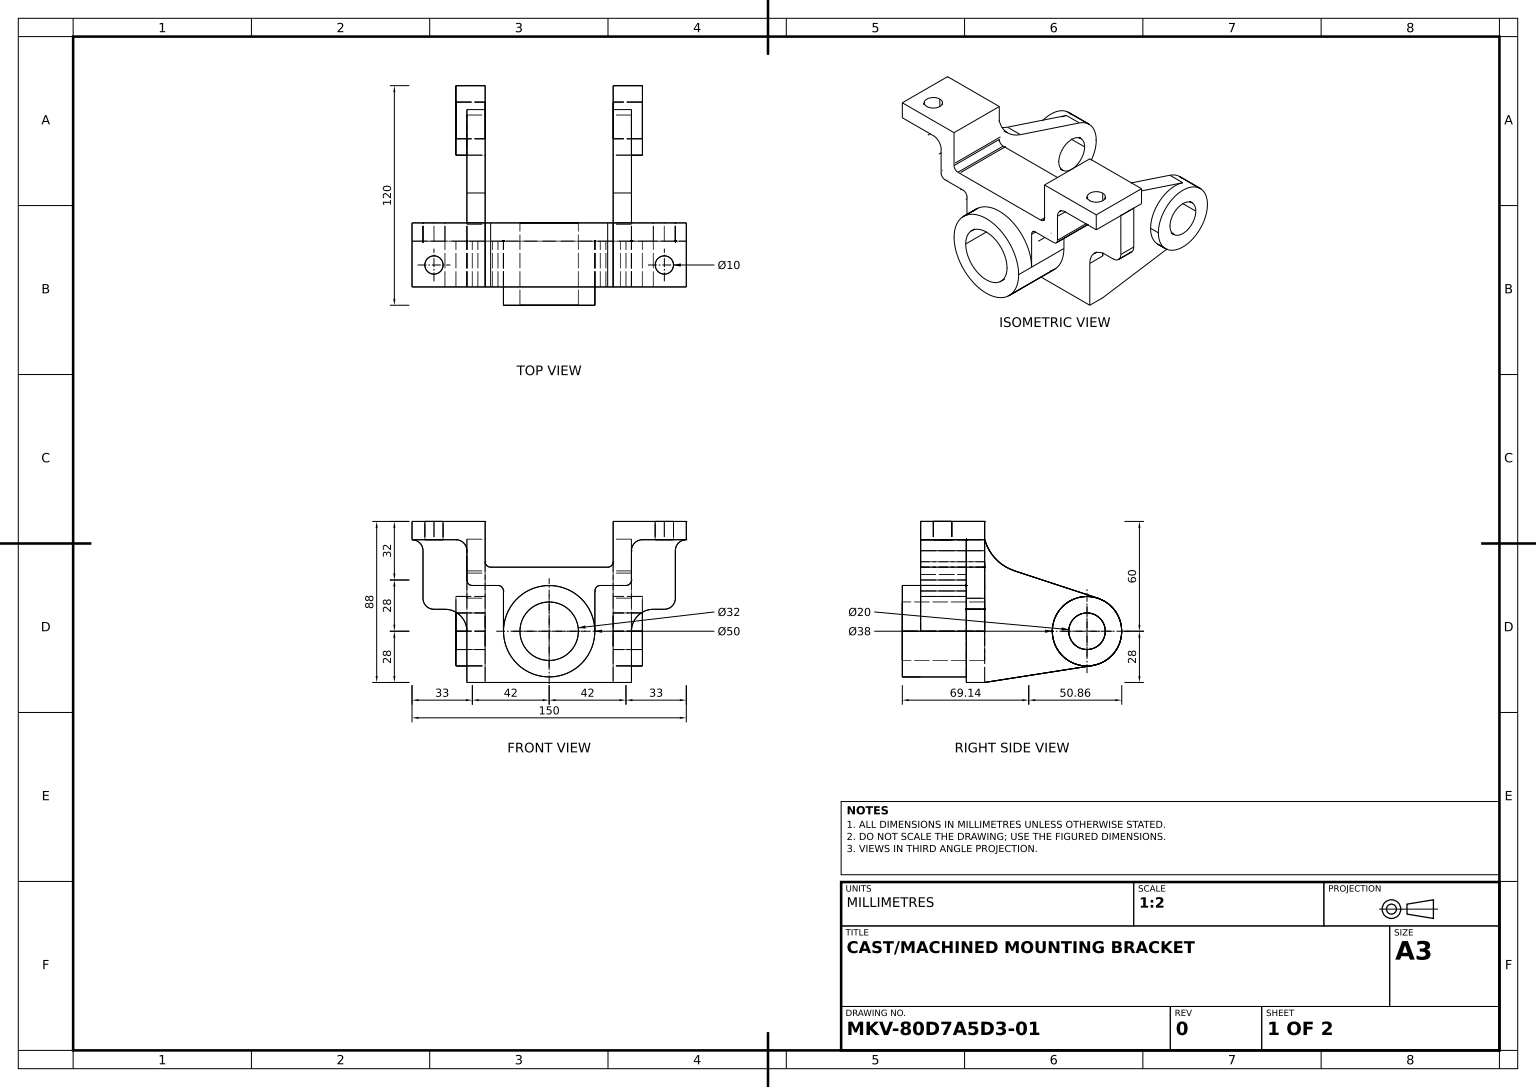
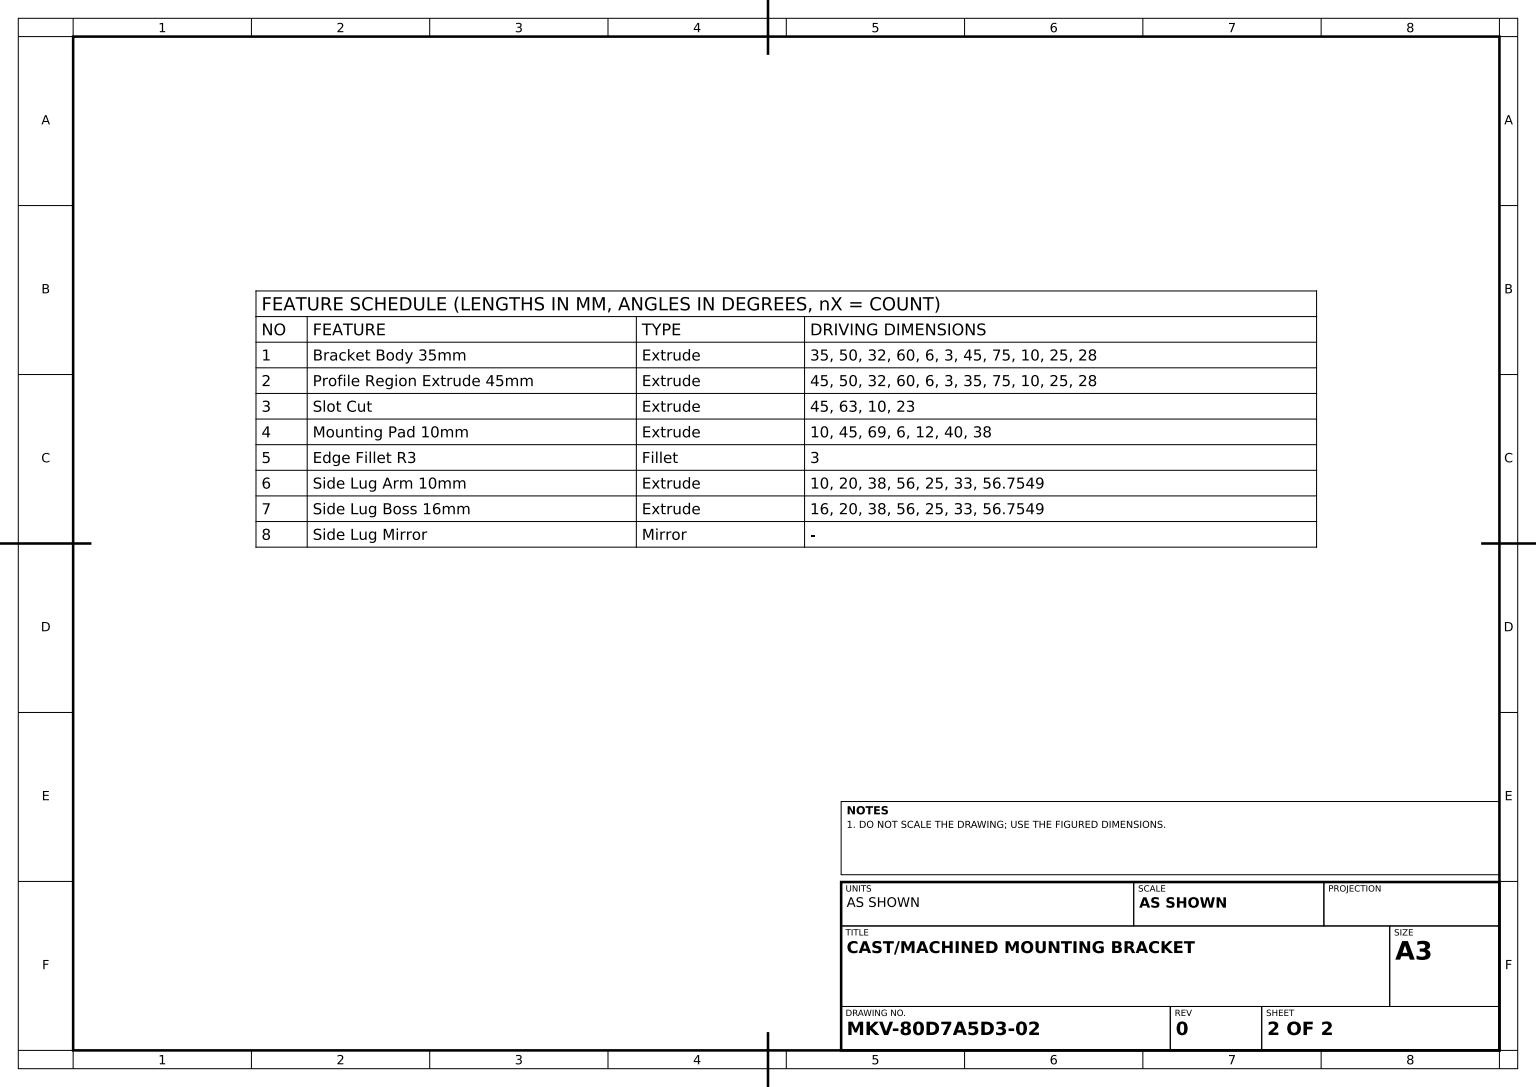
from build123d import *

# Parameters (mm, degrees)
BRACKET_BODY_35MM_DEPTH           = 35
PROFILE_REGION_EXTRUDE_45MM_DEPTH = 45
SLOT_CUT_SKETCH_R                 = 5
SLOT_CUT_DEPTH                    = 45
MOUNTING_PAD_10MM_DEPTH           = 10
EDGE_FILLET_R3_R                  = 3
SIDE_LUG_ARM_10MM_DEPTH           = 10
SKETCH6_3_R                       = 19
SKETCH6_3_R_2                     = 10
SIDE_LUG_BOSS_16MM_DEPTH          = 16


with BuildPart() as part:
    # Bracket Profile Sketch → Bracket Body 35mm (new body)
    with BuildSketch(Plane.XY):
        with BuildLine():
            Line((0, 35), (0, 25))
            ThreePointArc((0, 25), (17.67766953, 17.67766953), (25, 0))
            Line((25, 0), (25, 22))
            ThreePointArc((25, 22), (25.878679656, 24.121320344), (28, 25))
            Line((28, 25), (42, 25))
            ThreePointArc((42, 25), (44.121320344, 25.878679656), (45, 28))
            Line((45, 28), (45, 44))
            ThreePointArc((45, 44), (46.757359313, 48.242640687), (51, 50))
            Line((51, 50), (75, 50))
            Line((75, 50), (75, 60))
            Line((75, 60), (35, 60))
            Line((35, 60), (35, 35))
            Line((35, 35), (0, 35))
        make_face()
        with BuildLine():
            Line((-25, 22), (-25, 0))
            ThreePointArc((-25, 0), (-17.67766953, 17.67766953), (0, 25))
            Line((0, 25), (0, 35))
            Line((0, 35), (-35, 35))
            Line((-35, 35), (-35, 60))
            Line((-35, 60), (-75, 60))
            Line((-75, 60), (-75, 50))
            Line((-75, 50), (-51, 50))
            ThreePointArc((-51, 50), (-46.757359313, 48.242640687), (-45, 44))
            Line((-45, 44), (-45, 28))
            ThreePointArc((-45, 28), (-44.121320344, 25.878679656), (-42, 25))
            Line((-42, 25), (-28, 25))
            ThreePointArc((-28, 25), (-25.878679656, 24.121320344), (-25, 22))
        make_face()
    extrude(amount=BRACKET_BODY_35MM_DEPTH)

    # Sketch1_3 → Profile Region Extrude 45mm (add)
    with BuildSketch(Plane.XY):
        with BuildLine():
            ThreePointArc((0, 25), (-17.67766953, 17.67766953), (-25, 0))
            ThreePointArc((-25, 0), (-17.67766953, -17.67766953), (0, -25))
            Line((0, -25), (0, -16))
            ThreePointArc((0, -16), (-16, 0), (0, 16))
            Line((0, 16), (0, 25))
        make_face()
        with BuildLine():
            ThreePointArc((25, 0), (17.67766953, 17.67766953), (0, 25))
            Line((0, 25), (0, 16))
            ThreePointArc((0, 16), (11.313708499, 11.313708499), (16, 0))
            ThreePointArc((16, 0), (11.313708499, -11.313708499), (0, -16))
            Line((0, -16), (0, -25))
            ThreePointArc((0, -25), (17.67766953, -17.67766953), (25, 0))
        make_face()
        with BuildLine():
            ThreePointArc((0, 25), (-17.67766953, 17.67766953), (-25, 0))
            ThreePointArc((-25, 0), (-17.67766953, -17.67766953), (0, -25))
            Line((0, -25), (0, -16))
            ThreePointArc((0, -16), (-16, 0), (0, 16))
            Line((0, 16), (0, 25))
        make_face()
        with BuildLine():
            ThreePointArc((25, 0), (17.67766953, 17.67766953), (0, 25))
            Line((0, 25), (0, 16))
            ThreePointArc((0, 16), (11.313708499, 11.313708499), (16, 0))
            ThreePointArc((16, 0), (11.313708499, -11.313708499), (0, -16))
            Line((0, -16), (0, -25))
            ThreePointArc((0, -25), (17.67766953, -17.67766953), (25, 0))
        make_face()
    extrude(amount=PROFILE_REGION_EXTRUDE_45MM_DEPTH)

    # Slot Cut Sketch → Slot Cut (cut)
    with BuildSketch(Plane.XZ.offset(-50)):
        with Locations(Location((63, 23, 0), (0, 0, 270))):
            Circle(SLOT_CUT_SKETCH_R)
        with Locations(Location((-63, 23, 0), (0, 0, 270))):
            Circle(SLOT_CUT_SKETCH_R)
    extrude(amount=-SLOT_CUT_DEPTH, mode=Mode.SUBTRACT)

    # Mounting Pad Sketch → Mounting Pad 10mm (add)
    with BuildSketch(Plane(origin=(0, 0, 0), x_dir=(-1, 0, 0), z_dir=(0, 0, -1))):
        with BuildLine():
            Line((51, 50), (75, 50))
            ThreePointArc((75, 50), (70.757359313, 48.242640687), (69, 44))
            Line((69, 44), (69, 18))
            ThreePointArc((69, 18), (67.242640687, 13.757359313), (63, 12))
            Line((63, 12), (57, 12))
            ThreePointArc((57, 12), (48.514718626, 8.485281374), (45, 0))
            Line((45, 0), (45, -28))
            Line((45, -28), (-45, -28))
            Line((-45, -28), (-45, 0))
            ThreePointArc((-45, 0), (-48.514718626, 8.485281374), (-57, 12))
            Line((-57, 12), (-63, 12))
            ThreePointArc((-63, 12), (-67.242640687, 13.757359313), (-69, 18))
            Line((-69, 18), (-69, 44))
            ThreePointArc((-69, 44), (-70.757359313, 48.242640687), (-75, 50))
            Line((-75, 50), (-51, 50))
            ThreePointArc((-51, 50), (-46.757359313, 48.242640687), (-45, 44))
            Line((-45, 44), (-45, 28))
            ThreePointArc((-45, 28), (-44.121320344, 25.878679656), (-42, 25))
            Line((-42, 25), (-28, 25))
            ThreePointArc((-28, 25), (-25.878679656, 24.121320344), (-25, 22))
            Line((-25, 22), (-25, 0))
            ThreePointArc((-25, 0), (0, -25), (25, 0))
            Line((25, 0), (25, 22))
            ThreePointArc((25, 22), (25.878679656, 24.121320344), (28, 25))
            Line((28, 25), (42, 25))
            ThreePointArc((42, 25), (44.121320344, 25.878679656), (45, 28))
            Line((45, 28), (45, 44))
            ThreePointArc((45, 44), (46.757359313, 48.242640687), (51, 50))
        make_face()
    extrude(amount=-MOUNTING_PAD_10MM_DEPTH)

    # Edge Fillet R3
    edge_fillet_r3_edges = [part.edges().sort_by_distance(p)[0] for p in [
        (35, 35, 17.5),
        (-35, 35, 17.5),
    ]]
    fillet(edge_fillet_r3_edges, radius=EDGE_FILLET_R3_R)

    # Side Lug Sketch → Side Lug Arm 10mm (add)
    with BuildSketch(Plane(origin=(-35, 0, 0), x_dir=(0, 0, -1), z_dir=(1, 0, 0))):
        with BuildLine():
            ThreePointArc((58.939212458, -18.771282059), (37.062002462, 1.533704422), (61.921503767, 18.053691953))
            Line((61.921503767, 18.053691953), (16.35266654, 33))
            ThreePointArc((16.35266654, 33), (5.991213295, 39.565558274), (0, 50.269372176))
            Line((0, 50.269372176), (0, 38))
            Line((0, 38), (0, -28))
            Line((0, -28), (58.939212458, -18.771282059))
        make_face()
    side_lug_arm_10mm = extrude(amount=-SIDE_LUG_ARM_10MM_DEPTH)

    # Sketch6_3 → Side Lug Boss 16mm (add)
    with BuildSketch(Plane(origin=(-35, 0, 0), x_dir=(0, 0, -1), z_dir=(1, 0, 0))):
        with Locations((56, 0)):
            Circle(SKETCH6_3_R)
        with Locations((56, 0)):
            Circle(SKETCH6_3_R_2, mode=Mode.SUBTRACT)
    side_lug_boss_16mm = extrude(amount=-SIDE_LUG_BOSS_16MM_DEPTH)

    # Side Lug Mirror: Side Lug Arm 10mm, Side Lug Boss 16mm across plane
    add(side_lug_arm_10mm.mirror(Plane(origin=(0, 0, 0), x_dir=(0, 0, 1), z_dir=(1, 0, 0))))
    add(side_lug_boss_16mm.mirror(Plane(origin=(0, 0, 0), x_dir=(0, 0, 1), z_dir=(1, 0, 0))))


solid = part.part
